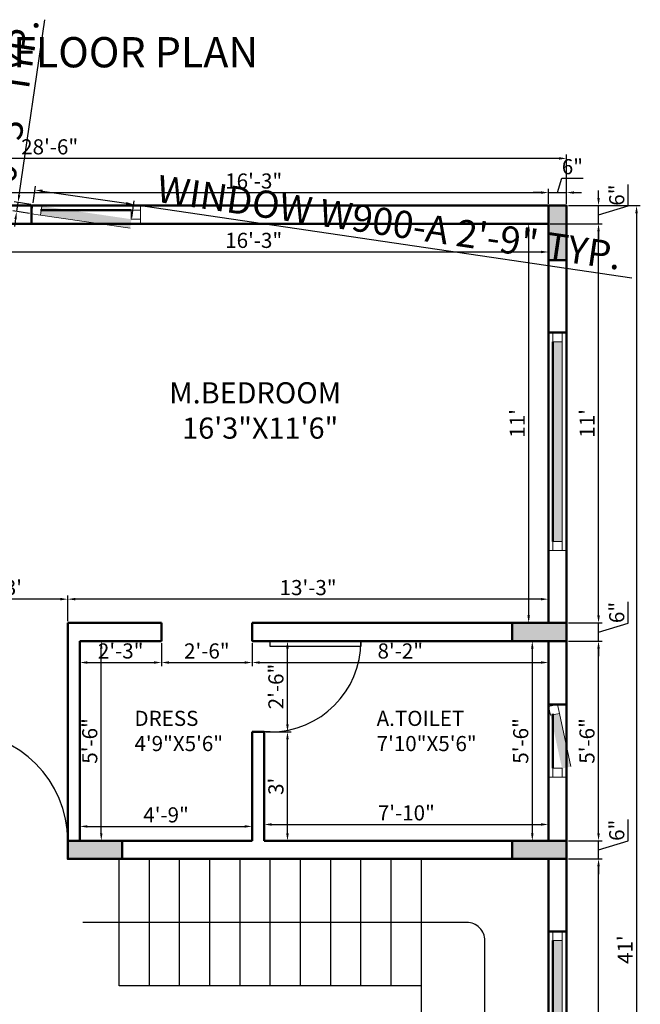
# Model space of a CAD drawing. Units: inches. Extents: x 3064 to 19385, y 846 to 15425.
# Tile 55 of 108: x 6630 to 6835, y 1132 to 1458. Entities that reach past the tile are written whole.
import ezdxf

# ---------------------------------------------------------------- set-up
doc = ezdxf.new("R2010")
doc.units = ezdxf.units.IN
for name, color, linetype, lineweight in [('A-ANNO-DIMS', 2, 'Continuous', 18), ('A-ANNO-TEXT', 7, 'Continuous', 25), ('A-AREA-IDEN', 3, 'Continuous', 18), ('A-COLS', 1, 'Continuous', 35), ('A-DOOR', 3, 'Continuous', 25), ('A-FLOR-STRS', 2, 'Continuous', 25), ('A-GLAZ', 4, 'Continuous', 18), ('A-WALL', 7, 'Continuous', 50)]:
    doc.layers.add(name, color=color, linetype=linetype, lineweight=lineweight)
doc.styles.get("Standard").update_dxf_attribs({"font": 'arial.ttf'})
doc.dimstyles.new('ISO-25', dxfattribs={"dimtxt": 9, "dimasz": 2.5, "dimexe": 1.25, "dimexo": 0.625, "dimtad": 1, "dimdec": 1, "dimlunit": 3, "dimtxsty": 'Standard', "dimcen": 2.5, "dimadec": 0, "dimazin": 0, "dimtfac": 1, "dimtdec": 1, "dimtmove": 0, "dimatfit": 3, "dimfxl": 1, "dimarcsym": 0})

# ---------------------------------------------------------------- blocks, each defined once
blk = doc.blocks.new('*U3')
for p, q in [((0, 0), (0, -6)), ((36, 0), (36, -6))]:
    blk.add_line(p, q)
blk.add_lwpolyline([(0, 0), (0, 36), (1.75, 36), (1.75, 0)], close=True)
blk.add_arc((0, 0), 36, 0, 90)
blk = doc.blocks.new('*U4')
for p, q in [((0, 0), (0, -6)), ((30, 0), (30, -6))]:
    blk.add_line(p, q)
blk.add_lwpolyline([(0, 0), (0, 30), (1.75, 30), (1.75, 0)], close=True)
blk.add_arc((0, 0), 30, 0, 90)
blk = doc.blocks.new('*D119')
at = {"layer": 'A-ANNO-DIMS', "color": 0, "lineweight": -2, "transparency": 16777216}
for p, q in [((6811.66, 1180.34), (6822.87, 1180.34)), ((6821.62, 984.84), (6821.62, 1177.84)), ((6805.66, 982.34), (6822.87, 982.34))]:
    blk.add_line(p, q, dxfattribs=at)
at = {"layer": 'A-ANNO-DIMS', "color": 0, "transparency": 16777216}
for points in [[(6821.2, 1177.84), (6822.03, 1177.84), (6821.62, 1180.34)], [(6821.2, 984.84), (6822.03, 984.84), (6821.62, 982.34)]]:
    blk.add_solid(points, dxfattribs=at)
at = {"layer": 'Defpoints', "color": 0, "transparency": 16777216}
for p in [(6811.03, 1180.34), (6821.62, 1180.34), (6805.03, 982.34)]:
    blk.add_point(p, dxfattribs=at)
at = {"layer": 'A-ANNO-DIMS', "color": 0, "transparency": 16777216, "insert": (6818.44, 1081.34), "char_height": 5, "attachment_point": 5, "rotation": 90}
blk.add_mtext('16\'-6"', dxfattribs=at)
blk = doc.blocks.new('*D120')
at = {"layer": 'A-ANNO-DIMS', "color": 0, "lineweight": -2, "transparency": 16777216}
for p, q in [((6831.46, 1186.29), (6831.46, 1193.32)), ((6821.62, 1188.84), (6821.62, 1191.34)), ((6811.66, 1186.34), (6822.87, 1186.34)), ((6821.62, 1180.34), (6821.62, 1186.34)), ((6821.62, 1180.34), (6821.62, 1186.34)), ((6821.62, 1183.34), (6831.46, 1186.29)), ((6811.66, 1180.34), (6822.87, 1180.34)), ((6821.62, 1177.84), (6821.62, 1175.34))]:
    blk.add_line(p, q, dxfattribs=at)
at = {"layer": 'A-ANNO-DIMS', "color": 0, "transparency": 16777216}
for points in [[(6821.2, 1188.84), (6822.03, 1188.84), (6821.62, 1186.34)], [(6821.2, 1177.84), (6822.03, 1177.84), (6821.62, 1180.34)]]:
    blk.add_solid(points, dxfattribs=at)
at = {"layer": 'Defpoints', "color": 0, "transparency": 16777216}
for p in [(6811.03, 1186.34), (6821.62, 1186.34), (6811.03, 1180.34)]:
    blk.add_point(p, dxfattribs=at)
at = {"layer": 'A-ANNO-DIMS', "color": 0, "transparency": 16777216, "insert": (6828.28, 1189.81), "char_height": 5, "attachment_point": 5, "rotation": 90}
blk.add_mtext('6"', dxfattribs=at)
blk = doc.blocks.new('*D121')
at = {"layer": 'A-ANNO-DIMS', "color": 0, "lineweight": -2, "transparency": 16777216}
for p, q in [((6811.66, 1252.34), (6822.87, 1252.34)), ((6821.62, 1188.84), (6821.62, 1249.84)), ((6811.66, 1186.34), (6822.87, 1186.34))]:
    blk.add_line(p, q, dxfattribs=at)
at = {"layer": 'A-ANNO-DIMS', "color": 0, "transparency": 16777216}
for points in [[(6821.2, 1249.84), (6822.03, 1249.84), (6821.62, 1252.34)], [(6821.2, 1188.84), (6822.03, 1188.84), (6821.62, 1186.34)]]:
    blk.add_solid(points, dxfattribs=at)
at = {"layer": 'Defpoints', "color": 0, "transparency": 16777216}
for p in [(6811.03, 1252.34), (6821.62, 1252.34), (6811.03, 1186.34)]:
    blk.add_point(p, dxfattribs=at)
at = {"layer": 'A-ANNO-DIMS', "color": 0, "transparency": 16777216, "insert": (6818.44, 1219.34), "char_height": 5, "attachment_point": 5, "rotation": 90}
blk.add_mtext('5\'-6"', dxfattribs=at)
blk = doc.blocks.new('*D122')
at = {"layer": 'A-ANNO-DIMS', "color": 0, "lineweight": -2, "transparency": 16777216}
for p, q in [((6821.62, 1260.84), (6821.62, 1263.34)), ((6831.46, 1258.29), (6831.46, 1265.32)), ((6811.66, 1258.34), (6822.87, 1258.34)), ((6821.62, 1252.34), (6821.62, 1258.34)), ((6821.62, 1252.34), (6821.62, 1258.34)), ((6821.62, 1255.34), (6831.46, 1258.29)), ((6811.66, 1252.34), (6822.87, 1252.34)), ((6821.62, 1249.84), (6821.62, 1247.34))]:
    blk.add_line(p, q, dxfattribs=at)
at = {"layer": 'A-ANNO-DIMS', "color": 0, "transparency": 16777216}
for points in [[(6821.2, 1260.84), (6822.03, 1260.84), (6821.62, 1258.34)], [(6821.2, 1249.84), (6822.03, 1249.84), (6821.62, 1252.34)]]:
    blk.add_solid(points, dxfattribs=at)
at = {"layer": 'Defpoints', "color": 0, "transparency": 16777216}
for p in [(6811.03, 1258.34), (6821.62, 1258.34), (6811.03, 1252.34)]:
    blk.add_point(p, dxfattribs=at)
at = {"layer": 'A-ANNO-DIMS', "color": 0, "transparency": 16777216, "insert": (6828.28, 1261.81), "char_height": 5, "attachment_point": 5, "rotation": 90}
blk.add_mtext('6"', dxfattribs=at)
blk = doc.blocks.new('*D102')
at = {"layer": 'A-ANNO-DIMS', "color": 0, "lineweight": -2, "transparency": 16777216}
for p, q in [((6805.66, 1390.34), (6822.87, 1390.34)), ((6821.62, 1260.84), (6821.62, 1387.84)), ((6811.66, 1258.34), (6822.87, 1258.34))]:
    blk.add_line(p, q, dxfattribs=at)
at = {"layer": 'A-ANNO-DIMS', "color": 0, "transparency": 16777216}
for points in [[(6821.2, 1387.84), (6822.03, 1387.84), (6821.62, 1390.34)], [(6821.2, 1260.84), (6822.03, 1260.84), (6821.62, 1258.34)]]:
    blk.add_solid(points, dxfattribs=at)
at = {"layer": 'Defpoints', "color": 0, "transparency": 16777216}
for p in [(6805.03, 1390.34), (6821.62, 1390.34), (6811.03, 1258.34)]:
    blk.add_point(p, dxfattribs=at)
at = {"layer": 'A-ANNO-DIMS', "color": 0, "transparency": 16777216, "insert": (6818.48, 1324.34), "char_height": 5, "attachment_point": 5, "rotation": 90}
blk.add_mtext("11'", dxfattribs=at)
blk = doc.blocks.new('*D103')
at = {"layer": 'A-ANNO-DIMS', "color": 0, "lineweight": -2, "transparency": 16777216}
for p, q in [((6831.46, 1396.29), (6831.46, 1403.32)), ((6821.62, 1398.84), (6821.62, 1401.34)), ((6811.66, 1396.34), (6822.87, 1396.34)), ((6821.62, 1390.34), (6821.62, 1396.34)), ((6821.62, 1390.34), (6821.62, 1396.34)), ((6821.62, 1393.34), (6831.46, 1396.29)), ((6805.66, 1390.34), (6822.87, 1390.34)), ((6821.62, 1387.84), (6821.62, 1385.34))]:
    blk.add_line(p, q, dxfattribs=at)
at = {"layer": 'A-ANNO-DIMS', "color": 0, "transparency": 16777216}
for points in [[(6821.2, 1398.84), (6822.03, 1398.84), (6821.62, 1396.34)], [(6821.2, 1387.84), (6822.03, 1387.84), (6821.62, 1390.34)]]:
    blk.add_solid(points, dxfattribs=at)
at = {"layer": 'Defpoints', "color": 0, "transparency": 16777216}
for p in [(6811.03, 1396.34), (6821.62, 1396.34), (6805.03, 1390.34)]:
    blk.add_point(p, dxfattribs=at)
at = {"layer": 'A-ANNO-DIMS', "color": 0, "transparency": 16777216, "insert": (6828.28, 1399.81), "char_height": 5, "attachment_point": 5, "rotation": 90}
blk.add_mtext('6"', dxfattribs=at)
blk = doc.blocks.new('*D104')
at = {"layer": 'A-ANNO-DIMS', "color": 0, "lineweight": -2, "transparency": 16777216}
for p, q in [((6811.66, 1396.34), (6835.44, 1396.34)), ((6834.19, 1393.84), (6834.19, 906.84)), ((6811.66, 904.34), (6835.44, 904.34))]:
    blk.add_line(p, q, dxfattribs=at)
at = {"layer": 'A-ANNO-DIMS', "color": 0, "transparency": 16777216}
for points in [[(6833.77, 1393.84), (6834.6, 1393.84), (6834.19, 1396.34)], [(6833.77, 906.84), (6834.6, 906.84), (6834.19, 904.34)]]:
    blk.add_solid(points, dxfattribs=at)
at = {"layer": 'Defpoints', "color": 0, "transparency": 16777216}
for p in [(6811.03, 1396.34), (6811.03, 904.34), (6834.19, 904.34)]:
    blk.add_point(p, dxfattribs=at)
at = {"layer": 'A-ANNO-DIMS', "color": 0, "transparency": 16777216, "insert": (6831.05, 1150.34), "char_height": 5, "attachment_point": 5, "rotation": 90}
blk.add_mtext("41'", dxfattribs=at)
blk = doc.blocks.new('*D100')
at = {"layer": 'A-ANNO-DIMS', "color": 0, "lineweight": -2, "transparency": 16777216}
for p, q in [((6610.03, 1396.96), (6610.03, 1401.9)), ((6612.53, 1400.65), (6802.53, 1400.65)), ((6805.03, 1396.96), (6805.03, 1401.9))]:
    blk.add_line(p, q, dxfattribs=at)
at = {"layer": 'A-ANNO-DIMS', "color": 0, "transparency": 16777216}
for points in [[(6612.53, 1401.07), (6612.53, 1400.24), (6610.03, 1400.65)], [(6802.53, 1401.07), (6802.53, 1400.24), (6805.03, 1400.65)]]:
    blk.add_solid(points, dxfattribs=at)
at = {"layer": 'Defpoints', "color": 0, "transparency": 16777216}
for p in [(6805.03, 1400.65), (6610.03, 1396.34), (6805.03, 1396.34)]:
    blk.add_point(p, dxfattribs=at)
at = {"layer": 'A-ANNO-DIMS', "color": 0, "transparency": 16777216, "insert": (6707.53, 1403.83), "char_height": 5, "attachment_point": 5}
blk.add_mtext('16\'-3"', dxfattribs=at)
blk = doc.blocks.new('*D101')
at = {"layer": 'A-ANNO-DIMS', "color": 0, "lineweight": -2, "transparency": 16777216}
for p, q in [((6808.03, 1400.65), (6809.46, 1405.39)), ((6809.46, 1405.39), (6816.48, 1405.39)), ((6802.53, 1400.65), (6800.03, 1400.65)), ((6805.03, 1396.96), (6805.03, 1401.9)), ((6805.03, 1400.65), (6811.03, 1400.65)), ((6805.03, 1400.65), (6811.03, 1400.65)), ((6811.03, 1396.96), (6811.03, 1401.9)), ((6813.53, 1400.65), (6816.03, 1400.65))]:
    blk.add_line(p, q, dxfattribs=at)
at = {"layer": 'A-ANNO-DIMS', "color": 0, "transparency": 16777216}
for points in [[(6802.53, 1401.07), (6802.53, 1400.24), (6805.03, 1400.65)], [(6813.53, 1401.07), (6813.53, 1400.24), (6811.03, 1400.65)]]:
    blk.add_solid(points, dxfattribs=at)
at = {"layer": 'Defpoints', "color": 0, "transparency": 16777216}
for p in [(6811.03, 1400.65), (6805.03, 1396.34), (6811.03, 1396.34)]:
    blk.add_point(p, dxfattribs=at)
at = {"layer": 'A-ANNO-DIMS', "color": 0, "transparency": 16777216, "insert": (6812.97, 1408.57), "char_height": 5, "attachment_point": 5}
blk.add_mtext('6"', dxfattribs=at)
blk = doc.blocks.new('*D96')
at = {"layer": 'A-ANNO-DIMS', "color": 0, "lineweight": -2, "transparency": 16777216}
for p, q in [((6469.03, 1396.96), (6469.03, 1413.2)), ((6811.03, 1396.96), (6811.03, 1413.2)), ((6808.53, 1411.95), (6471.53, 1411.95))]:
    blk.add_line(p, q, dxfattribs=at)
at = {"layer": 'A-ANNO-DIMS', "color": 0, "transparency": 16777216}
for points in [[(6471.53, 1412.37), (6471.53, 1411.53), (6469.03, 1411.95)], [(6808.53, 1412.37), (6808.53, 1411.53), (6811.03, 1411.95)]]:
    blk.add_solid(points, dxfattribs=at)
at = {"layer": 'Defpoints', "color": 0, "transparency": 16777216}
for p in [(6469.03, 1411.95), (6469.03, 1396.34), (6811.03, 1396.34)]:
    blk.add_point(p, dxfattribs=at)
at = {"layer": 'A-ANNO-DIMS', "color": 0, "transparency": 16777216, "insert": (6640.03, 1415.13), "char_height": 5, "attachment_point": 5}
blk.add_mtext('28\'-6"', dxfattribs=at)
blk = doc.blocks.new('*D203')
at = {"layer": 'A-ANNO-DIMS', "color": 0, "lineweight": -2, "transparency": 16777216}
for p, q in [((6650.66, 1252.34), (6658.36, 1252.34)), ((6657.11, 1188.84), (6657.11, 1249.84)), ((6650.66, 1186.34), (6658.36, 1186.34))]:
    blk.add_line(p, q, dxfattribs=at)
at = {"layer": 'A-ANNO-DIMS', "color": 0, "transparency": 16777216}
for points in [[(6656.7, 1249.84), (6657.53, 1249.84), (6657.11, 1252.34)], [(6656.7, 1188.84), (6657.53, 1188.84), (6657.11, 1186.34)]]:
    blk.add_solid(points, dxfattribs=at)
at = {"layer": 'Defpoints', "color": 0, "transparency": 16777216}
for p in [(6650.03, 1252.34), (6657.11, 1252.34), (6650.03, 1186.34)]:
    blk.add_point(p, dxfattribs=at)
at = {"layer": 'A-ANNO-DIMS', "color": 0, "transparency": 16777216, "insert": (6653.94, 1219.34), "char_height": 5, "attachment_point": 5, "rotation": 90}
blk.add_mtext('5\'-6"', dxfattribs=at)
blk = doc.blocks.new('*D204')
at = {"layer": 'A-ANNO-DIMS', "color": 0, "lineweight": -2, "transparency": 16777216}
for p, q in [((6650.03, 1186.96), (6650.03, 1192.33)), ((6707.03, 1186.96), (6707.03, 1192.33)), ((6652.53, 1191.08), (6704.53, 1191.08))]:
    blk.add_line(p, q, dxfattribs=at)
at = {"layer": 'A-ANNO-DIMS', "color": 0, "transparency": 16777216}
for points in [[(6652.53, 1191.49), (6652.53, 1190.66), (6650.03, 1191.08)], [(6704.53, 1191.49), (6704.53, 1190.66), (6707.03, 1191.08)]]:
    blk.add_solid(points, dxfattribs=at)
at = {"layer": 'Defpoints', "color": 0, "transparency": 16777216}
for p in [(6707.03, 1191.08), (6650.03, 1186.34), (6707.03, 1186.34)]:
    blk.add_point(p, dxfattribs=at)
at = {"layer": 'A-ANNO-DIMS', "color": 0, "transparency": 16777216, "insert": (6678.53, 1194.25), "char_height": 5, "attachment_point": 5}
blk.add_mtext('4\'-9"', dxfattribs=at)
blk = doc.blocks.new('*D205')
at = {"layer": 'A-ANNO-DIMS', "color": 0, "lineweight": -2, "transparency": 16777216}
for p, q in [((6711.03, 1186.96), (6711.03, 1192.98)), ((6713.53, 1191.73), (6802.53, 1191.73)), ((6805.03, 1186.96), (6805.03, 1192.98))]:
    blk.add_line(p, q, dxfattribs=at)
at = {"layer": 'A-ANNO-DIMS', "color": 0, "transparency": 16777216}
for points in [[(6713.53, 1192.15), (6713.53, 1191.31), (6711.03, 1191.73)], [(6802.53, 1192.15), (6802.53, 1191.31), (6805.03, 1191.73)]]:
    blk.add_solid(points, dxfattribs=at)
at = {"layer": 'Defpoints', "color": 0, "transparency": 16777216}
for p in [(6805.03, 1191.73), (6711.03, 1186.34), (6805.03, 1186.34)]:
    blk.add_point(p, dxfattribs=at)
at = {"layer": 'A-ANNO-DIMS', "color": 0, "transparency": 16777216, "insert": (6758.03, 1194.91), "char_height": 5, "attachment_point": 5}
blk.add_mtext('7\'-10"', dxfattribs=at)
blk = doc.blocks.new('*D206')
at = {"layer": 'A-ANNO-DIMS', "color": 0, "lineweight": -2, "transparency": 16777216}
for p, q in [((6804.41, 1252.34), (6798.45, 1252.34)), ((6799.7, 1249.84), (6799.7, 1188.84)), ((6804.41, 1186.34), (6798.45, 1186.34))]:
    blk.add_line(p, q, dxfattribs=at)
at = {"layer": 'A-ANNO-DIMS', "color": 0, "transparency": 16777216}
for points in [[(6799.28, 1249.84), (6800.12, 1249.84), (6799.7, 1252.34)], [(6799.28, 1188.84), (6800.12, 1188.84), (6799.7, 1186.34)]]:
    blk.add_solid(points, dxfattribs=at)
at = {"layer": 'Defpoints', "color": 0, "transparency": 16777216}
for p in [(6805.03, 1252.34), (6799.7, 1186.34), (6805.03, 1186.34)]:
    blk.add_point(p, dxfattribs=at)
at = {"layer": 'A-ANNO-DIMS', "color": 0, "transparency": 16777216, "insert": (6796.52, 1219.34), "char_height": 5, "attachment_point": 5, "rotation": 90}
blk.add_mtext('5\'-6"', dxfattribs=at)
blk = doc.blocks.new('*D207')
at = {"layer": 'A-ANNO-DIMS', "color": 0, "lineweight": -2, "transparency": 16777216}
for p, q in [((6711.66, 1222.34), (6719.96, 1222.34)), ((6718.71, 1188.84), (6718.71, 1219.84)), ((6711.66, 1186.34), (6719.96, 1186.34))]:
    blk.add_line(p, q, dxfattribs=at)
at = {"layer": 'A-ANNO-DIMS', "color": 0, "transparency": 16777216}
for points in [[(6718.29, 1219.84), (6719.13, 1219.84), (6718.71, 1222.34)], [(6718.29, 1188.84), (6719.13, 1188.84), (6718.71, 1186.34)]]:
    blk.add_solid(points, dxfattribs=at)
at = {"layer": 'Defpoints', "color": 0, "transparency": 16777216}
for p in [(6711.03, 1222.34), (6718.71, 1222.34), (6711.03, 1186.34)]:
    blk.add_point(p, dxfattribs=at)
at = {"layer": 'A-ANNO-DIMS', "color": 0, "transparency": 16777216, "insert": (6715.53, 1204.34), "char_height": 5, "attachment_point": 5, "rotation": 90}
blk.add_mtext("3'", dxfattribs=at)
blk = doc.blocks.new('*D208')
at = {"layer": 'A-ANNO-DIMS', "color": 0, "lineweight": -2, "transparency": 16777216}
for p, q in [((6719.34, 1252.34), (6719.96, 1252.34)), ((6718.71, 1224.84), (6718.71, 1249.84)), ((6711.66, 1222.34), (6719.96, 1222.34))]:
    blk.add_line(p, q, dxfattribs=at)
at = {"layer": 'A-ANNO-DIMS', "color": 0, "transparency": 16777216}
for points in [[(6718.29, 1249.84), (6719.13, 1249.84), (6718.71, 1252.34)], [(6718.29, 1224.84), (6719.13, 1224.84), (6718.71, 1222.34)]]:
    blk.add_solid(points, dxfattribs=at)
at = {"layer": 'Defpoints', "color": 0, "transparency": 16777216}
for p in [(6718.71, 1252.34), (6718.71, 1252.34), (6711.03, 1222.34)]:
    blk.add_point(p, dxfattribs=at)
at = {"layer": 'A-ANNO-DIMS', "color": 0, "transparency": 16777216, "insert": (6715.53, 1237.34), "char_height": 5, "attachment_point": 5, "rotation": 90}
blk.add_mtext('2\'-6"', dxfattribs=at)
blk = doc.blocks.new('*D209')
at = {"layer": 'A-ANNO-DIMS', "color": 0, "lineweight": -2, "transparency": 16777216}
for p, q in [((6650.03, 1251.71), (6650.03, 1244.02)), ((6677.03, 1251.71), (6677.03, 1244.02)), ((6652.53, 1245.27), (6674.53, 1245.27))]:
    blk.add_line(p, q, dxfattribs=at)
at = {"layer": 'A-ANNO-DIMS', "color": 0, "transparency": 16777216}
for points in [[(6652.53, 1245.69), (6652.53, 1244.86), (6650.03, 1245.27)], [(6674.53, 1245.69), (6674.53, 1244.86), (6677.03, 1245.27)]]:
    blk.add_solid(points, dxfattribs=at)
at = {"layer": 'Defpoints', "color": 0, "transparency": 16777216}
for p in [(6650.03, 1252.34), (6677.03, 1252.34), (6677.03, 1245.27)]:
    blk.add_point(p, dxfattribs=at)
at = {"layer": 'A-ANNO-DIMS', "color": 0, "transparency": 16777216, "insert": (6663.53, 1248.45), "char_height": 5, "attachment_point": 5}
blk.add_mtext('2\'-3"', dxfattribs=at)
blk = doc.blocks.new('*D210')
at = {"layer": 'A-ANNO-DIMS', "color": 0, "lineweight": -2, "transparency": 16777216}
for p, q in [((6677.03, 1251.71), (6677.03, 1244.02)), ((6707.03, 1251.71), (6707.03, 1244.02)), ((6679.53, 1245.27), (6704.53, 1245.27))]:
    blk.add_line(p, q, dxfattribs=at)
at = {"layer": 'A-ANNO-DIMS', "color": 0, "transparency": 16777216}
for points in [[(6679.53, 1245.69), (6679.53, 1244.86), (6677.03, 1245.27)], [(6704.53, 1245.69), (6704.53, 1244.86), (6707.03, 1245.27)]]:
    blk.add_solid(points, dxfattribs=at)
at = {"layer": 'Defpoints', "color": 0, "transparency": 16777216}
for p in [(6677.03, 1252.34), (6707.03, 1252.34), (6707.03, 1245.27)]:
    blk.add_point(p, dxfattribs=at)
at = {"layer": 'A-ANNO-DIMS', "color": 0, "transparency": 16777216, "insert": (6692.03, 1248.45), "char_height": 5, "attachment_point": 5}
blk.add_mtext('2\'-6"', dxfattribs=at)
blk = doc.blocks.new('*D211')
at = {"layer": 'A-ANNO-DIMS', "color": 0, "lineweight": -2, "transparency": 16777216}
for p, q in [((6707.03, 1251.71), (6707.03, 1244.02)), ((6805.03, 1251.71), (6805.03, 1244.02)), ((6709.53, 1245.27), (6802.53, 1245.27))]:
    blk.add_line(p, q, dxfattribs=at)
at = {"layer": 'A-ANNO-DIMS', "color": 0, "transparency": 16777216}
for points in [[(6709.53, 1245.69), (6709.53, 1244.86), (6707.03, 1245.27)], [(6802.53, 1245.69), (6802.53, 1244.86), (6805.03, 1245.27)]]:
    blk.add_solid(points, dxfattribs=at)
at = {"layer": 'Defpoints', "color": 0, "transparency": 16777216}
for p in [(6707.03, 1252.34), (6805.03, 1252.34), (6805.03, 1245.27)]:
    blk.add_point(p, dxfattribs=at)
at = {"layer": 'A-ANNO-DIMS', "color": 0, "transparency": 16777216, "insert": (6756.03, 1248.45), "char_height": 5, "attachment_point": 5}
blk.add_mtext('8\'-2"', dxfattribs=at)
blk = doc.blocks.new('*D212')
at = {"layer": 'A-ANNO-DIMS', "color": 0, "lineweight": -2, "transparency": 16777216}
for p, q in [((6610.03, 1389.71), (6610.03, 1379.77)), ((6805.03, 1389.71), (6805.03, 1379.77)), ((6612.53, 1381.02), (6802.53, 1381.02))]:
    blk.add_line(p, q, dxfattribs=at)
at = {"layer": 'A-ANNO-DIMS', "color": 0, "transparency": 16777216}
for points in [[(6612.53, 1381.44), (6612.53, 1380.6), (6610.03, 1381.02)], [(6802.53, 1381.44), (6802.53, 1380.6), (6805.03, 1381.02)]]:
    blk.add_solid(points, dxfattribs=at)
at = {"layer": 'Defpoints', "color": 0, "transparency": 16777216}
for p in [(6610.03, 1390.34), (6805.03, 1390.34), (6805.03, 1381.02)]:
    blk.add_point(p, dxfattribs=at)
at = {"layer": 'A-ANNO-DIMS', "color": 0, "transparency": 16777216, "insert": (6707.53, 1384.2), "char_height": 5, "attachment_point": 5}
blk.add_mtext('16\'-3"', dxfattribs=at)
blk = doc.blocks.new('*D213')
at = {"layer": 'A-ANNO-DIMS', "color": 0, "lineweight": -2, "transparency": 16777216}
for p, q in [((6804.41, 1390.34), (6797.25, 1390.34)), ((6798.5, 1387.84), (6798.5, 1260.84)), ((6804.41, 1258.34), (6797.25, 1258.34))]:
    blk.add_line(p, q, dxfattribs=at)
at = {"layer": 'A-ANNO-DIMS', "color": 0, "transparency": 16777216}
for points in [[(6798.09, 1387.84), (6798.92, 1387.84), (6798.5, 1390.34)], [(6798.09, 1260.84), (6798.92, 1260.84), (6798.5, 1258.34)]]:
    blk.add_solid(points, dxfattribs=at)
at = {"layer": 'Defpoints', "color": 0, "transparency": 16777216}
for p in [(6805.03, 1390.34), (6798.5, 1258.34), (6805.03, 1258.34)]:
    blk.add_point(p, dxfattribs=at)
at = {"layer": 'A-ANNO-DIMS', "color": 0, "transparency": 16777216, "insert": (6795.37, 1324.34), "char_height": 5, "attachment_point": 5, "rotation": 90}
blk.add_mtext("11'", dxfattribs=at)
blk = doc.blocks.new('*D214')
at = {"layer": 'A-ANNO-DIMS', "color": 0, "lineweight": -2, "transparency": 16777216}
for p, q in [((6646.03, 1258.96), (6646.03, 1267.47)), ((6805.03, 1258.96), (6805.03, 1267.47)), ((6802.53, 1266.22), (6648.53, 1266.22))]:
    blk.add_line(p, q, dxfattribs=at)
at = {"layer": 'A-ANNO-DIMS', "color": 0, "transparency": 16777216}
for points in [[(6648.53, 1266.64), (6648.53, 1265.81), (6646.03, 1266.22)], [(6802.53, 1266.64), (6802.53, 1265.81), (6805.03, 1266.22)]]:
    blk.add_solid(points, dxfattribs=at)
at = {"layer": 'Defpoints', "color": 0, "transparency": 16777216}
for p in [(6646.03, 1266.22), (6646.03, 1258.34), (6805.03, 1258.34)]:
    blk.add_point(p, dxfattribs=at)
at = {"layer": 'A-ANNO-DIMS', "color": 0, "transparency": 16777216, "insert": (6725.53, 1269.4), "char_height": 5, "attachment_point": 5}
blk.add_mtext('13\'-3"', dxfattribs=at)
blk = doc.blocks.new('*D215')
at = {"layer": 'A-ANNO-DIMS', "color": 0, "lineweight": -2, "transparency": 16777216}
for p, q in [((6610.03, 1269.71), (6610.03, 1264.97)), ((6646.03, 1258.96), (6646.03, 1267.47)), ((6643.53, 1266.22), (6612.53, 1266.22))]:
    blk.add_line(p, q, dxfattribs=at)
at = {"layer": 'A-ANNO-DIMS', "color": 0, "transparency": 16777216}
for points in [[(6612.53, 1266.64), (6612.53, 1265.81), (6610.03, 1266.22)], [(6643.53, 1266.64), (6643.53, 1265.81), (6646.03, 1266.22)]]:
    blk.add_solid(points, dxfattribs=at)
at = {"layer": 'Defpoints', "color": 0, "transparency": 16777216}
for p in [(6610.03, 1270.34), (6610.03, 1266.22), (6646.03, 1258.34)]:
    blk.add_point(p, dxfattribs=at)
at = {"layer": 'A-ANNO-DIMS', "color": 0, "transparency": 16777216, "insert": (6628.03, 1269.4), "char_height": 5, "attachment_point": 5}
blk.add_mtext("3'", dxfattribs=at)
blk = doc.blocks.new('WIN-900-A')
h = blk.add_hatch(color=256)
h.dxf.hatch_style = 1
h.paths.add_polyline_path([(33, 0), (33, 3), (3, 3), (3, 0)])
blk.add_line((3, 0), (33, 0))
blk.add_lwpolyline([(3, 0), (0, 0), (0, 3), (3, 3)], close=True)
blk = doc.blocks.new('WIN-600')
h = blk.add_hatch(color=256)
h.dxf.hatch_style = 1
h.paths.add_polyline_path([(3, 18), (0, 18), (0, 0), (3, 0)])
blk.add_line((3, 18), (3, 0))
blk.add_lwpolyline([(3, 18), (0, 18), (0, 21), (3, 21)], close=True)
blk = doc.blocks.new('WIN-1800-PAIR')
h = blk.add_hatch(color=256)
h.dxf.hatch_style = 1
h.paths.add_polyline_path([(0, 0), (3, 0), (3, 70.5), (0, 70.5)])
h.paths.add_polyline_path([(3, 144), (0, 144), (0, 73.5), (3, 73.5)])
blk.add_line((3, 144), (3, 73.5))
blk.add_lwpolyline([(3, 144), (0, 144), (0, 147), (3, 147)], close=True)
blk = doc.blocks.new('WIN-1900')
blk.add_line((3, 0), (3, 66))
blk.add_lwpolyline([(3, 66), (0, 66), (0, 69), (3, 69)], close=True)
blk = doc.blocks.new('*D437')
at = {"layer": 'A-ANNO-DIMS', "color": 0, "lineweight": -2, "transparency": 16777216}
for p, q in [((6634.55, 1397.26), (6635.36, 1402.77)), ((6637.65, 1401.17), (6665.35, 1397.1)), ((6667.2, 1392.45), (6668.01, 1397.97)), ((6667.83, 1396.73), (6832.6, 1372.5))]:
    blk.add_line(p, q, dxfattribs=at)
at = {"layer": 'A-ANNO-DIMS', "color": 0, "transparency": 16777216}
for points in [[(6637.71, 1401.58), (6637.59, 1400.76), (6635.18, 1401.53)], [(6665.41, 1397.51), (6665.29, 1396.69), (6667.83, 1396.73)]]:
    blk.add_solid(points, dxfattribs=at)
at = {"layer": 'Defpoints', "color": 0, "transparency": 16777216}
for p in [(6634.46, 1396.64), (6667.83, 1396.73), (6667.11, 1391.84)]:
    blk.add_point(p, dxfattribs=at)
at = {"layer": 'A-ANNO-DIMS', "color": 0, "transparency": 16777216, "insert": (6752.22, 1389.66), "char_height": 9, "attachment_point": 5, "rotation": 351.6351}
blk.add_mtext('WINDOW W900-A 2\'-9" TYP.', dxfattribs=at)
blk = doc.blocks.new('*D438')
at = {"layer": 'A-ANNO-DIMS', "color": 0, "lineweight": -2, "transparency": 16777216}
for p, q in [((6629.92, 1399.83), (6638.45, 1457.82)), ((6633.84, 1396.73), (6628.32, 1397.54)), ((6629.12, 1394.39), (6629.56, 1397.36)), ((6633.4, 1393.76), (6627.89, 1394.57)), ((6628.76, 1391.92), (6628.4, 1389.44))]:
    blk.add_line(p, q, dxfattribs=at)
at = {"layer": 'A-ANNO-DIMS', "color": 0, "transparency": 16777216}
for points in [[(6629.51, 1399.89), (6630.34, 1399.77), (6629.56, 1397.36)], [(6628.35, 1391.98), (6629.17, 1391.86), (6629.12, 1394.39)]]:
    blk.add_solid(points, dxfattribs=at)
at = {"layer": 'Defpoints', "color": 0, "transparency": 16777216}
for p in [(6629.56, 1397.36), (6634.46, 1396.64), (6634.02, 1393.67)]:
    blk.add_point(p, dxfattribs=at)
at = {"layer": 'A-ANNO-DIMS', "color": 0, "transparency": 16777216, "insert": (6629.2, 1430.82), "char_height": 9, "attachment_point": 5, "rotation": 81.6351}
blk.add_mtext('0\'-3" TYP.', dxfattribs=at)

msp = doc.modelspace()

# ---------------------------------------------------------------- hatches: boundary and pattern name
at = {"layer": 'A-COLS'}
h = msp.add_hatch(color=256, dxfattribs=at)
h.dxf.hatch_style = 1
h.paths.add_polyline_path([(6805.03, 1378.34), (6811.03, 1378.34), (6811.03, 1396.34), (6805.03, 1396.34)])
h = msp.add_hatch(color=256, dxfattribs=at)
h.dxf.hatch_style = 1
h.paths.add_polyline_path([(6811.03, 1252.34), (6811.03, 1258.34), (6793.03, 1258.34), (6793.03, 1252.34)])
h = msp.add_hatch(color=256, dxfattribs=at)
h.dxf.hatch_style = 1
h.paths.add_polyline_path([(6664.03, 1180.34), (6664.03, 1186.34), (6646.03, 1186.34), (6646.03, 1180.34)])
h = msp.add_hatch(color=256, dxfattribs=at)
h.dxf.hatch_style = 1
h.paths.add_polyline_path([(6811.03, 1180.34), (6811.03, 1186.34), (6793.03, 1186.34), (6793.03, 1180.34)])
at = {"layer": 'A-GLAZ'}
h = msp.add_hatch(color=256, dxfattribs=at)
h.dxf.hatch_style = 1
h.paths.add_polyline_path([(6806.53, 1285.34), (6809.53, 1285.34), (6809.53, 1351.34), (6806.53, 1351.34)])

# ---------------------------------------------------------------- linework, layer by layer
at = {"layer": 'A-FLOR-STRS'}
for p, q in [((6663.03, 1138.34), (6663.03, 1180.34)), ((6673.03, 1138.34), (6673.03, 1180.34)), ((6683.03, 1138.34), (6683.03, 1180.34)), ((6693.03, 1138.34), (6693.03, 1180.34)), ((6703.03, 1138.34), (6703.03, 1180.34)), ((6713.03, 1138.34), (6713.03, 1180.34)), ((6723.03, 1138.34), (6723.03, 1180.34)), ((6733.03, 1138.34), (6733.03, 1180.34)), ((6743.03, 1138.34), (6743.03, 1180.34)), ((6753.03, 1138.34), (6753.03, 1180.34)), ((6763.03, 1024.34), (6763.03, 1180.34)), ((6763.03, 1138.34), (6663.03, 1138.34))]:
    msp.add_line(p, q, dxfattribs=at)
msp.add_lwpolyline([(6670.52, 1003.34), (6778.03, 1003.34, 0.414214), (6784.03, 1009.34), (6784.03, 1153.34, 0.414214), (6778.03, 1159.34), (6651.03, 1159.34)], format="xyb", dxfattribs=at)
at = {"layer": 'A-GLAZ'}
for p, q in [((6670.03, 1396.34), (6670.03, 1390.34)), ((6811.03, 1282.34), (6805.03, 1282.34)), ((6805.03, 1207.34), (6811.03, 1207.34))]:
    msp.add_line(p, q, dxfattribs=at)
for points in [[(6670.03, 1391.84), (6667.03, 1391.84), (6667.03, 1394.84), (6670.03, 1394.84)], [(6809.53, 1282.34), (6806.53, 1282.34), (6806.53, 1285.34), (6809.53, 1285.34)], [(6809.53, 1207.34), (6806.53, 1207.34), (6806.53, 1210.34), (6809.53, 1210.34)]]:
    msp.add_lwpolyline(points, close=True, dxfattribs=at)
at = {"layer": 'A-WALL'}
for p, q in [((6811.03, 1396.34), (6469.03, 1396.34)), ((6634.03, 1396.34), (6634.03, 1390.34)), ((6637.03, 1394.84), (6667.03, 1394.84)), ((6811.03, 904.34), (6811.03, 1396.34)), ((6805.03, 1390.34), (6610.03, 1390.34)), ((6805.03, 1258.34), (6805.03, 1390.34)), ((6805.03, 1354.34), (6811.03, 1354.34)), ((6806.53, 1351.34), (6806.53, 1285.34)), ((6677.03, 1258.34), (6646.03, 1258.34)), ((6646.03, 1258.34), (6646.03, 1180.34)), ((6677.03, 1258.34), (6677.03, 1252.34)), ((6805.03, 1258.34), (6707.03, 1258.34)), ((6707.03, 1258.34), (6707.03, 1252.34)), ((6677.03, 1252.34), (6650.03, 1252.34)), ((6650.03, 1252.34), (6650.03, 1186.34)), ((6805.03, 1252.34), (6707.03, 1252.34)), ((6805.03, 1186.34), (6805.03, 1252.34)), ((6805.03, 1231.34), (6811.03, 1231.34)), ((6806.53, 1228.34), (6806.53, 1210.34)), ((6711.03, 1222.34), (6707.03, 1222.34)), ((6707.03, 1222.34), (6707.03, 1186.34)), ((6711.03, 1186.34), (6711.03, 1222.34)), ((6707.03, 1186.34), (6650.03, 1186.34)), ((6805.03, 1186.34), (6711.03, 1186.34)), ((6805.03, 1180.34), (6646.03, 1180.34)), ((6805.03, 982.34), (6805.03, 1180.34)), ((6811.03, 1156.34), (6805.03, 1156.34)), ((6806.53, 1153.34), (6806.53, 1082.84))]:
    msp.add_line(p, q, dxfattribs=at)
for points in [[(6811.03, 1378.34), (6811.03, 1396.34), (6805.03, 1396.34), (6805.03, 1378.34)], [(6811.03, 1258.34), (6793.03, 1258.34), (6793.03, 1252.34), (6811.03, 1252.34)], [(6664.03, 1186.34), (6646.03, 1186.34), (6646.03, 1180.34), (6664.03, 1180.34)], [(6811.03, 1186.34), (6793.03, 1186.34), (6793.03, 1180.34), (6811.03, 1180.34)]]:
    msp.add_lwpolyline(points, close=True, dxfattribs=at)

# ---------------------------------------------------------------- block references
at = {"layer": 'A-DOOR', "rotation": 270}
msp.add_blockref('*U4', (6713.03, 1252.34), dxfattribs=at)
at = {"layer": 'A-DOOR'}
msp.add_blockref('*U3', (6610.03, 1186.34), dxfattribs=at)
at = {"layer": 'A-GLAZ'}
for name, p, rotation in [('WIN-900-A', (6634.02, 1393.67), 351.6350998303231), ('WIN-600', (6809.54, 1210.23), 12.21571913413082)]:
    msp.add_blockref(name, p, dxfattribs=dict(at, rotation=rotation))
for name, p in [('WIN-1900', (6806.53, 1285.34)), ('WIN-1800-PAIR', (6806.53, 1009.34))]:
    msp.add_blockref(name, p, dxfattribs=at)

# ---------------------------------------------------------------- texts
at = {"layer": 'A-ANNO-TEXT', "insert": (6588.38, 1452.06), "char_height": 10, "attachment_point": 1}
msp.add_mtext_dynamic_manual_height_columns('FIRST FLOOR PLAN', width=200.9739, gutter_width=12.5, heights=[0], dxfattribs=at)
at = {"layer": 'A-AREA-IDEN', "attachment_point": 1}
for s, insert, char_height in [('M.BEDROOM\\P  16\'3"X11\'6"', (6679.59, 1337.94), 7), ('DRESS\\P4\'9"X5\'6"', (6668.08, 1229.31), 5), ('A.TOILET\\P7\'10"X5\'6"', (6748.2, 1229.31), 5)]:
    msp.add_mtext_dynamic_manual_height_columns(s, width=67.5924, gutter_width=12.5, heights=[0], dxfattribs=dict(at, insert=insert, char_height=char_height))

# ---------------------------------------------------------------- dimensions: what is measured, and where the dimension line sits
at = {"layer": 'A-ANNO-DIMS'}
for base, p1, p2, angle, text, picture, middle in [((6629.56, 1397.36), (6634.02, 1393.67), (6634.46, 1396.64), 81.6351, '<> TYP.', '*D438', (6629.2, 1430.82)), ((6667.83, 1396.73), (6634.46, 1396.64), (6667.11, 1391.84), 351.6351, 'WINDOW W900-A <> TYP.', '*D437', (6752.22, 1389.66))]:
    dim = msp.add_linear_dim(base=base, p1=p1, p2=p2, angle=angle, text=text, dimstyle='ISO-25', override={"dimdec": 1, "dimrnd": 0, "dimzin": 1, "dimlunit": 4, "dimfrac": 2}, dxfattribs=at)
    dim.commit()
    dim.dimension.update_dxf_attribs({"geometry": picture, "text_midpoint": middle})
for base, p1, p2, override, picture, middle in [((6469.03, 1411.95), (6811.03, 1396.34), (6469.03, 1396.34), {"dimtxt": 5, "dimclrd": 0, "dimclre": 0, "dimclrt": 0}, '*D96', (6640.03, 1415.13)), ((6811.03, 1400.65), (6805.03, 1396.34), (6811.03, 1396.34), {"dimtxt": 5, "dimclrd": 0, "dimclre": 0, "dimclrt": 0, "dimtmove": 1}, '*D101', (6810.08, 1408.57)), ((6805.03, 1400.65), (6610.03, 1396.34), (6805.03, 1396.34), {"dimtxt": 5, "dimclrd": 0, "dimclre": 0, "dimclrt": 0, "dimtmove": 1}, '*D100', (6707.53, 1403.83)), ((6805.03, 1381.02), (6610.03, 1390.34), (6805.03, 1390.34), {"dimtxt": 5, "dimclrd": 0, "dimclre": 0, "dimclrt": 0}, '*D212', (6707.53, 1384.2)), ((6610.03, 1266.22), (6646.03, 1258.34), (6610.03, 1270.34), {"dimtxt": 5, "dimclrd": 0, "dimclre": 0, "dimclrt": 0, "dimtmove": 1}, '*D215', (6628.03, 1269.4)), ((6646.03, 1266.22), (6805.03, 1258.34), (6646.03, 1258.34), {"dimtxt": 5, "dimclrd": 0, "dimclre": 0, "dimclrt": 0}, '*D214', (6725.53, 1269.4)), ((6677.03, 1245.27), (6650.03, 1252.34), (6677.03, 1252.34), {"dimtxt": 5, "dimclrd": 0, "dimclre": 0, "dimclrt": 0}, '*D209', (6663.53, 1248.45)), ((6707.03, 1245.27), (6677.03, 1252.34), (6707.03, 1252.34), {"dimtxt": 5, "dimclrd": 0, "dimclre": 0, "dimclrt": 0, "dimtmove": 1}, '*D210', (6692.03, 1248.45)), ((6805.03, 1245.27), (6707.03, 1252.34), (6805.03, 1252.34), {"dimtxt": 5, "dimclrd": 0, "dimclre": 0, "dimclrt": 0, "dimtmove": 1}, '*D211', (6756.03, 1248.45)), ((6805.03, 1191.73), (6711.03, 1186.34), (6805.03, 1186.34), {"dimtxt": 5, "dimclrd": 0, "dimclre": 0, "dimclrt": 0}, '*D205', (6758.03, 1194.91)), ((6707.03, 1191.08), (6650.03, 1186.34), (6707.03, 1186.34), {"dimtxt": 5, "dimclrd": 0, "dimclre": 0, "dimclrt": 0}, '*D204', (6678.53, 1194.25))]:
    dim = msp.add_linear_dim(base=base, p1=p1, p2=p2, dimstyle='ISO-25', override=override, dxfattribs=at)
    dim.commit()
    dim.dimension.update_dxf_attribs({"geometry": picture, "text_midpoint": middle})
for base, p1, p2, override, picture, middle in [((6821.62, 1396.34), (6805.03, 1390.34), (6811.03, 1396.34), {"dimtxt": 5, "dimclrd": 0, "dimclre": 0, "dimclrt": 0, "dimtmove": 1}, '*D103', (6828.28, 1396.92)), ((6834.19, 904.34), (6811.03, 1396.34), (6811.03, 904.34), {"dimtxt": 5, "dimclrd": 0, "dimclre": 0, "dimclrt": 0}, '*D104', (6831.05, 1150.34)), ((6798.5, 1258.34), (6805.03, 1390.34), (6805.03, 1258.34), {"dimtxt": 5, "dimclrd": 0, "dimclre": 0, "dimclrt": 0}, '*D213', (6795.37, 1324.34)), ((6821.62, 1390.34), (6811.03, 1258.34), (6805.03, 1390.34), {"dimtxt": 5, "dimclrd": 0, "dimclre": 0, "dimclrt": 0, "dimtmove": 1}, '*D102', (6818.48, 1324.34)), ((6821.62, 1258.34), (6811.03, 1252.34), (6811.03, 1258.34), {"dimtxt": 5, "dimclrd": 0, "dimclre": 0, "dimclrt": 0, "dimtmove": 1}, '*D122', (6828.28, 1258.92)), ((6657.11, 1252.34), (6650.03, 1186.34), (6650.03, 1252.34), {"dimtxt": 5, "dimclrd": 0, "dimclre": 0, "dimclrt": 0}, '*D203', (6653.94, 1219.34)), ((6718.71, 1252.34), (6711.03, 1222.34), (6718.71, 1252.34), {"dimtxt": 5, "dimclrd": 0, "dimclre": 0, "dimclrt": 0, "dimtmove": 1}, '*D208', (6715.53, 1237.34)), ((6799.7, 1186.34), (6805.03, 1252.34), (6805.03, 1186.34), {"dimtxt": 5, "dimclrd": 0, "dimclre": 0, "dimclrt": 0}, '*D206', (6796.52, 1219.34)), ((6821.62, 1252.34), (6811.03, 1186.34), (6811.03, 1252.34), {"dimtxt": 5, "dimclrd": 0, "dimclre": 0, "dimclrt": 0, "dimtmove": 1}, '*D121', (6818.44, 1219.34)), ((6718.71, 1222.34), (6711.03, 1186.34), (6711.03, 1222.34), {"dimtxt": 5, "dimclrd": 0, "dimclre": 0, "dimclrt": 0}, '*D207', (6715.53, 1204.34)), ((6821.62, 1186.34), (6811.03, 1180.34), (6811.03, 1186.34), {"dimtxt": 5, "dimclrd": 0, "dimclre": 0, "dimclrt": 0, "dimtmove": 1}, '*D120', (6828.28, 1186.92)), ((6821.62, 1180.34), (6805.03, 982.34), (6811.03, 1180.34), {"dimtxt": 5, "dimclrd": 0, "dimclre": 0, "dimclrt": 0, "dimtmove": 1}, '*D119', (6818.44, 1081.34))]:
    dim = msp.add_linear_dim(base=base, p1=p1, p2=p2, angle=90, dimstyle='ISO-25', override=override, dxfattribs=at)
    dim.commit()
    dim.dimension.update_dxf_attribs({"geometry": picture, "text_midpoint": middle})

doc.saveas('drawing.dxf')
